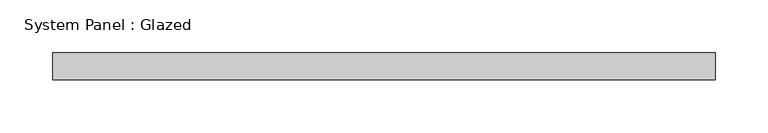
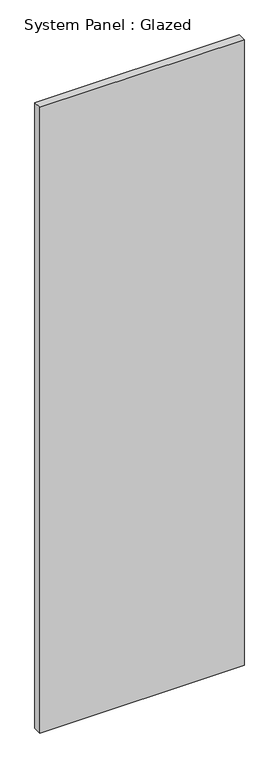
"""IFC4 building model written with IfcOpenShell, lengths in millimetres: plate geometry, System Panel : Glazed."""

from ifc_helpers import new_model, si_unit, origin, origin_with_axes, place, context, project, spatial, polyline, outline, extrude, source, transform, mapped, element, save


def system_panel_glazed_8ed2b2ee(model_context):
    return source(origin(), model_context, "Body", "SweptSolid", [
        extrude(outline(polyline([(313.8552609, 19.05), (-313.8552609, 19.05), (-313.8552609, 44.45), (313.8552609, 44.45), (313.8552609, 19.05)])), origin_with_axes(), (0.0, 0.0, 1.0), 2032.0),
    ])


if __name__ == "__main__":
    model = new_model("IFC4")
    model_context = context("Model", 3, world=origin())
    ifc_project = project(units=[si_unit("LENGTHUNIT", "METRE", prefix="MILLI")], contexts=[model_context])
    site = spatial("IfcSite", under=ifc_project)
    building = spatial("IfcBuilding", under=site)
    placement = place(None, origin())
    system_panel_glazed_shape = system_panel_glazed_8ed2b2ee(model_context)
    element("IfcPlate", 1, ObjectType="System Panel : Glazed", at=placement, inside=building, context=model_context, shape_type="MappedRepresentation", body=[
        mapped(system_panel_glazed_shape, transform((0.0, 0.0, 0.0), x_axis=(1.0, 0.0, 0.0), y_axis=(0.0, 1.0, 0.0), z_axis=(0.0, 0.0, 1.0))),
    ])
    save(model, "model.ifc")

# Revit data of these elements
# Type "System Panel : Glazed"
#   Construction Type Id = "GSP4R"
#   Analytic Construction = "1/8 in Pilkington single glazing"
#   Visual Light Transmittance = 0.9
#   Solar Heat Gain Coefficient = 0.86
#   Heat Transfer Coefficient (U) = 1.18115 BTU/(h·ft²·°F)
# Element 1 (IfcPlate, "System Panel : Glazed")
#   Materials on its faces: "Glass"
# Materials
#   "Glass": class "Glass", colour RGB 0 128 192, transparency 0.75, Description = "Soda Lime Glass", Cost = 0
